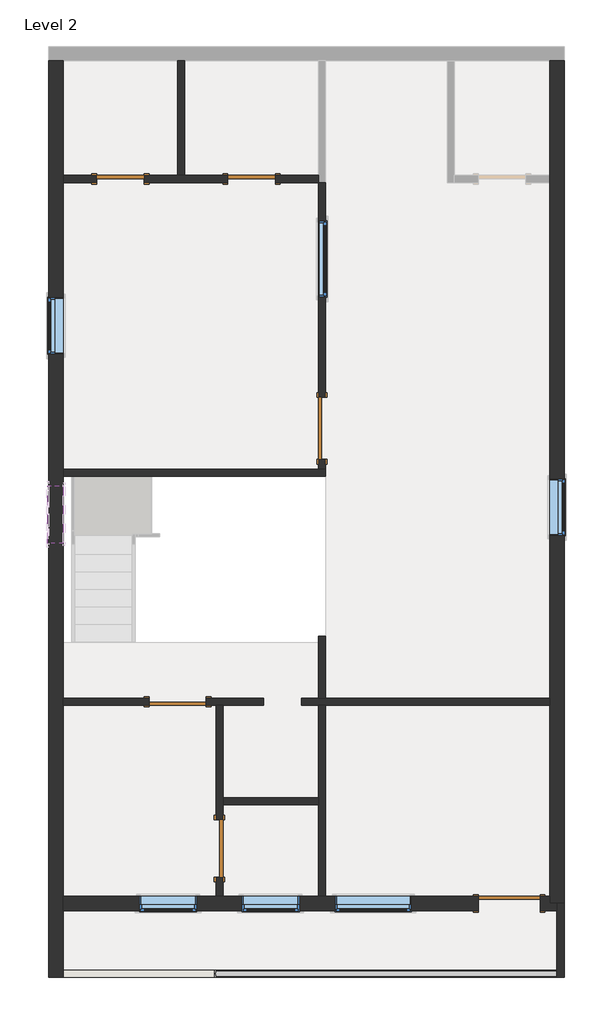
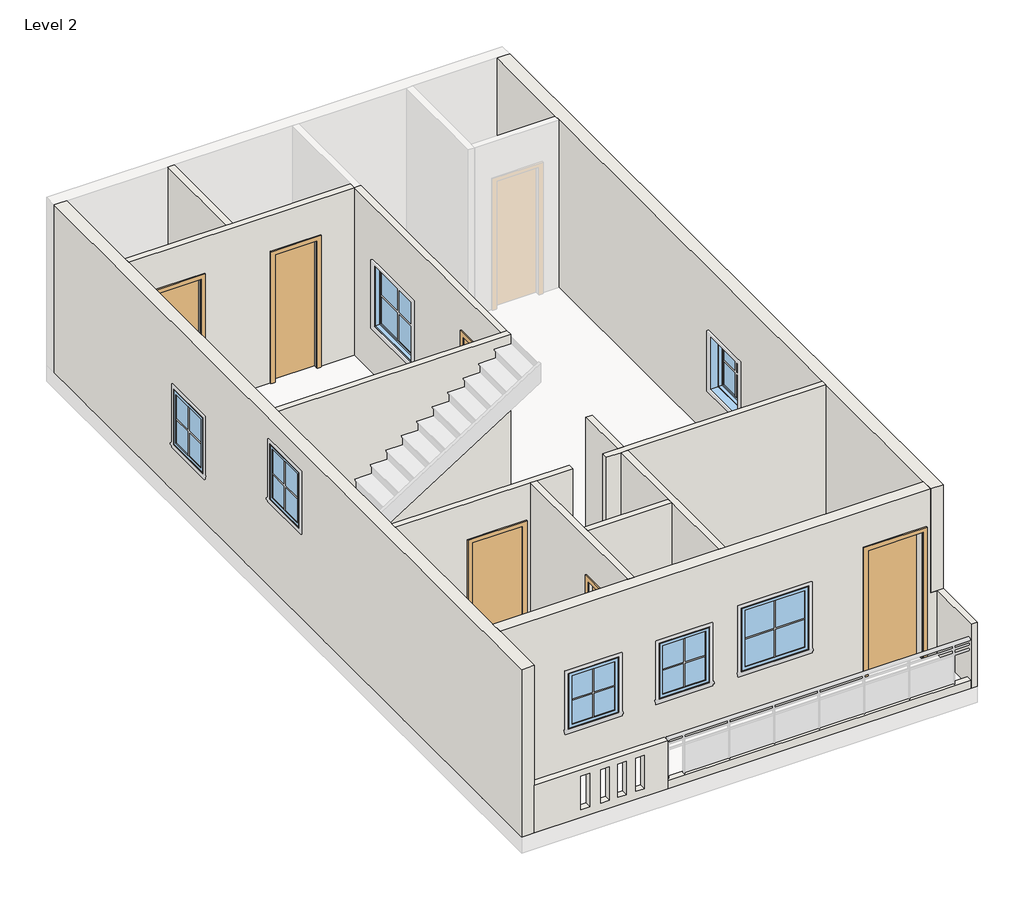
# One storey, part 1 of 2: 15 walls, 7 windows, 6 doors.
"""IFC4 building model written with IfcOpenShell, lengths in millimetres."""

from ifc_helpers import new_model, si_unit, frame, origin, place, context, project, spatial, polyline, outline, extrude, faceted_brep, transform, mapped, element, save
from components import door_02e7543a, door_3ddad2be, single_flush_d2_3_x_7_58d0fc15, door_c9b15bbd, door_019bc352, window_casement_single_left_w_4_x_4_e869003f, window_casement_single_left_w_4_x_4_9640c864, window_cb922c77, window_a1546d9a

model = new_model("IFC4")

# Units and contexts
model_context = context("Model", 3, world=origin())
ifc_project = project(units=[si_unit("LENGTHUNIT", "METRE", prefix="MILLI")], contexts=[model_context])

# Site, building, storey
site = spatial("IfcSite", under=ifc_project)
building = spatial("IfcBuilding", under=site)
storey = spatial("IfcBuildingStorey", under=building, Name="Level 2", Elevation=3200.4)

# Doors
placement = place(None, origin())
door_shape = door_02e7543a(model_context)
element("IfcDoor", 1, ObjectType="Single-Flush : D1 3'3\" X 7'", at=placement, inside=storey, context=model_context, shape_type="MappedRepresentation", body=[
    mapped(door_shape, transform((-6568.6167709, -3138.8637867, 3200.4), x_axis=(1.0, 0.0, 0.0), y_axis=(0.0, 1.0, 0.0), z_axis=(0.0, 0.0, 1.0))),
])
door_2_shape = door_3ddad2be(model_context)
element("IfcDoor", 2, ObjectType="Single-Flush : D1 3'3\" X 7'", at=placement, inside=storey, context=model_context, shape_type="MappedRepresentation", body=[
    mapped(door_2_shape, transform((-9559.4667709, 4443.0362133, 3200.4), x_axis=(0.0, -1.0, 0.0), y_axis=(1.0, 0.0, 0.0), z_axis=(0.0, 0.0, 1.0))),
])
single_flush_d2_3_x_7_shape = single_flush_d2_3_x_7_58d0fc15(model_context)
element("IfcDoor", 3, ObjectType="Single-Flush : D2 3' X 7'", at=placement, inside=storey, context=model_context, shape_type="MappedRepresentation", body=[
    mapped(single_flush_d2_3_x_7_shape, transform((-11864.5167709, 80.5862133, 3200.4), x_axis=(1.0, 0.0, 0.0), y_axis=(0.0, 1.0, 0.0), z_axis=(0.0, 0.0, 1.0))),
])
element("IfcDoor", 4, ObjectType="Single-Flush : D2 3' X 7'", at=placement, inside=storey, context=model_context, shape_type="MappedRepresentation", body=[
    mapped(single_flush_d2_3_x_7_shape, transform((-11197.7667709, -2262.5637867, 3200.4), x_axis=(0.0, 1.0, 0.0), y_axis=(-1.0, 0.0, 0.0), z_axis=(0.0, 0.0, 1.0))),
])
door_3_shape = door_c9b15bbd(model_context)
element("IfcDoor", 5, ObjectType="Single-Flush : D3 2'6\" X 7'", at=placement, inside=storey, context=model_context, shape_type="MappedRepresentation", body=[
    mapped(door_3_shape, transform((-12778.9167709, 8424.4862133, 3200.4), x_axis=(1.0, 0.0, 0.0), y_axis=(0.0, 1.0, 0.0), z_axis=(0.0, 0.0, 1.0))),
])
door_4_shape = door_019bc352(model_context)
element("IfcDoor", 6, ObjectType="Single-Flush : D3 2'6\" X 7'", at=placement, inside=storey, context=model_context, shape_type="MappedRepresentation", body=[
    mapped(door_4_shape, transform((-10683.4167709, 8424.4862133, 3200.4), x_axis=(-1.0, 0.0, 0.0), y_axis=(0.0, -1.0, 0.0), z_axis=(0.0, 0.0, 1.0))),
])

# Walls
element("IfcWall", 7, ObjectType="4.5\" inner wall", at=placement, inside=storey, context=model_context, shape_type="SweptSolid", body=[
    extrude(outline(polyline([(-11864.5167709, 8481.6362133), (-11864.5167709, 10310.4362133), (-11750.2167709, 10310.4362133), (-11750.2167709, 8481.6362133), (-11864.5167709, 8481.6362133)])), frame((0.0, 0.0, 3200.4), z_axis=(0.0, 0.0, 1.0), x_axis=(1.0, 0.0, 0.0)), (0.0, 0.0, 1.0), 3200.4),
])
element("IfcWall", 8, ObjectType="4.5\" inner wall", at=placement, inside=storey, context=model_context, shape_type="Brep", body=[
    faceted_brep([(-11064.4167709, 8481.6362133, 5638.8), (-11064.4167709, 8481.6362133, 3200.4), (-11750.2167709, 8481.6362133, 3200.4), (-11864.5167709, 8481.6362133, 3200.4), (-12397.9167709, 8481.6362133, 3200.4), (-12397.9167709, 8481.6362133, 5638.8), (-13159.9167709, 8481.6362133, 5638.8), (-13159.9167709, 8481.6362133, 3200.4), (-13693.3167709, 8481.6362133, 3200.4), (-13693.3167709, 8481.6362133, 6400.8), (-11864.5167709, 8481.6362133, 6400.8), (-11750.2167709, 8481.6362133, 6400.8), (-9616.6167709, 8481.6362133, 6400.8), (-9616.6167709, 8481.6362133, 3200.4), (-10302.4167709, 8481.6362133, 3200.4), (-10302.4167709, 8481.6362133, 5638.8), (-12397.9167709, 8367.3362133, 3200.4), (-11064.4167709, 8367.3362133, 3200.4), (-11064.4167709, 8367.3362133, 5638.8), (-10302.4167709, 8367.3362133, 5638.8), (-10302.4167709, 8367.3362133, 3200.4), (-9616.6167709, 8367.3362133, 3200.4), (-9616.6167709, 8367.3362133, 6400.8), (-13693.3167709, 8367.3362133, 6400.8), (-13693.3167709, 8367.3362133, 3200.4), (-13159.9167709, 8367.3362133, 3200.4), (-13159.9167709, 8367.3362133, 5638.8), (-12397.9167709, 8367.3362133, 5638.8)], [[[0, 1, 2, 3, 4, 5, 6, 7, 8, 9, 10, 11, 12, 13, 14, 15]], [[16, 17, 18, 19, 20, 21, 22, 23, 24, 25, 26, 27]], [[25, 24, 8, 7]], [[14, 13, 21, 20]], [[4, 3, 2, 1, 17, 16]], [[12, 11, 10, 9, 23, 22]], [[9, 8, 24, 23]], [[13, 12, 22, 21]], [[5, 4, 16, 27]], [[6, 5, 27, 26]], [[7, 6, 26, 25]], [[18, 17, 1, 0]], [[19, 18, 0, 15]], [[20, 19, 15, 14]]]),
])
element("IfcWall", 9, ObjectType="4.5\" inner wall", at=placement, inside=storey, context=model_context, shape_type="Brep", body=[
    faceted_brep([(-13693.3167709, 3681.0362133, 3200.4), (-9502.3167709, 3681.0362133, 3200.4), (-9502.3167709, 3681.0362133, 6400.8), (-13693.3167709, 3681.0362133, 6400.8), (-13693.3167709, 3795.3362133, 3200.4), (-13693.3167709, 3795.3362133, 6400.8), (-9616.6167709, 3795.3362133, 6400.8), (-9502.3167709, 3795.3362133, 6400.8), (-9502.3167709, 3795.3362133, 3200.4), (-9616.6167709, 3795.3362133, 3200.4)], [[[0, 1, 2, 3]], [[4, 5, 6, 7, 8, 9]], [[1, 0, 4, 9, 8]], [[3, 2, 7, 6, 5]], [[0, 3, 5, 4]], [[2, 1, 8, 7]]]),
])
element("IfcWall", 10, ObjectType="4.5\" inner wall", at=placement, inside=storey, context=model_context, shape_type="SweptSolid", body=[
    extrude(outline(polyline([(3947.7362133, 5638.8), (3947.7362133, 3200.4), (3795.3362133, 3200.4), (3795.3362133, 6400.8), (8367.3362133, 6400.8), (8367.3362133, 3200.4), (4938.3362133, 3200.4), (4938.3362133, 5638.8), (3947.7362133, 5638.8)]), holes=[polyline([(6538.5362133, 5334.0), (6538.5362133, 4114.8), (7757.7362133, 4114.8), (7757.7362133, 5334.0), (6538.5362133, 5334.0)])]), frame((-9616.6167709, 0.0, 0.0), z_axis=(1.0, 0.0, 0.0), x_axis=(0.0, 1.0, 0.0)), (0.0, 0.0, 1.0), 114.3),
])
element("IfcWall", 11, ObjectType="4.5\" inner wall", at=placement, inside=storey, context=model_context, shape_type="Brep", body=[
    faceted_brep([(-11407.3167709, 23.4362133, 5638.8), (-11407.3167709, 23.4362133, 3200.4), (-11254.9167709, 23.4362133, 3200.4), (-11140.6167709, 23.4362133, 3200.4), (-10492.9167709, 23.4362133, 3200.4), (-10492.9167709, 23.4362133, 6400.8), (-11140.6167709, 23.4362133, 6400.8), (-11254.9167709, 23.4362133, 6400.8), (-13693.3167709, 23.4362133, 6400.8), (-13693.3167709, 23.4362133, 3200.4), (-12321.7167709, 23.4362133, 3200.4), (-12321.7167709, 23.4362133, 5638.8), (-10492.9167709, 137.7362133, 3200.4), (-11407.3167709, 137.7362133, 3200.4), (-11407.3167709, 137.7362133, 5638.8), (-12321.7167709, 137.7362133, 5638.8), (-12321.7167709, 137.7362133, 3200.4), (-13693.3167709, 137.7362133, 3200.4), (-13693.3167709, 137.7362133, 6400.8), (-10492.9167709, 137.7362133, 6400.8)], [[[0, 1, 2, 3, 4, 5, 6, 7, 8, 9, 10, 11]], [[12, 13, 14, 15, 16, 17, 18, 19]], [[10, 9, 17, 16]], [[4, 3, 2, 1, 13, 12]], [[5, 4, 12, 19]], [[8, 7, 6, 5, 19, 18]], [[9, 8, 18, 17]], [[14, 13, 1, 0]], [[15, 14, 0, 11]], [[16, 15, 11, 10]]]),
])
element("IfcWall", 12, ObjectType="4.5\" inner wall", at=placement, inside=storey, context=model_context, shape_type="Brep", body=[
    faceted_brep([(-11254.9167709, 23.4362133, 3200.4), (-11254.9167709, -1805.3637867, 3200.4), (-11254.9167709, -1805.3637867, 5638.8), (-11254.9167709, -2719.7637867, 5638.8), (-11254.9167709, -2719.7637867, 3200.4), (-11254.9167709, -3024.5637867, 3200.4), (-11254.9167709, -3024.5637867, 6400.8), (-11254.9167709, 23.4362133, 6400.8), (-11140.6167709, -1805.3637867, 5638.8), (-11140.6167709, -1805.3637867, 3200.4), (-11140.6167709, -1564.0637867, 3200.4), (-11140.6167709, -1449.7637867, 3200.4), (-11140.6167709, 23.4362133, 3200.4), (-11140.6167709, 23.4362133, 6400.8), (-11140.6167709, -1449.7637867, 6400.8), (-11140.6167709, -1564.0637867, 6400.8), (-11140.6167709, -3024.5637867, 6400.8), (-11140.6167709, -3024.5637867, 3200.4), (-11140.6167709, -2719.7637867, 3200.4), (-11140.6167709, -2719.7637867, 5638.8)], [[[0, 1, 2, 3, 4, 5, 6, 7]], [[8, 9, 10, 11, 12, 13, 14, 15, 16, 17, 18, 19]], [[18, 17, 5, 4]], [[12, 11, 10, 9, 1, 0]], [[7, 6, 16, 15, 14, 13]], [[6, 5, 17, 16]], [[0, 7, 13, 12]], [[2, 1, 9, 8]], [[3, 2, 8, 19]], [[4, 3, 19, 18]]]),
])
element("IfcWall", 13, ObjectType="4.5\" inner wall", at=placement, inside=storey, context=model_context, shape_type="Brep", body=[
    faceted_brep([(-9502.3167709, 1128.3362133, 3200.4), (-9502.3167709, 1128.3362133, 6400.8), (-9502.3167709, 137.7362133, 6400.8), (-9502.3167709, 137.7362133, 3200.4), (-9616.6167709, 1128.3362133, 6400.8), (-9616.6167709, 1128.3362133, 3200.4), (-9616.6167709, 137.7362133, 3200.4), (-9616.6167709, 137.7362133, 6400.8)], [[[0, 1, 2, 3]], [[4, 5, 6, 7]], [[5, 0, 3, 6]], [[1, 0, 5, 4]], [[1, 4, 7, 2]], [[3, 2, 7, 6]]]),
    faceted_brep([(-9502.3167709, -3024.5637867, 6400.8), (-9502.3167709, -3024.5637867, 3200.4), (-9502.3167709, 23.4362133, 3200.4), (-9502.3167709, 23.4362133, 6400.8), (-9616.6167709, -3024.5637867, 3200.4), (-9616.6167709, -3024.5637867, 6400.8), (-9616.6167709, -1564.0637867, 6400.8), (-9616.6167709, -1449.7637867, 6400.8), (-9616.6167709, 23.4362133, 6400.8), (-9616.6167709, 23.4362133, 3200.4), (-9616.6167709, -1449.7637867, 3200.4), (-9616.6167709, -1564.0637867, 3200.4)], [[[0, 1, 2, 3]], [[4, 5, 6, 7, 8, 9, 10, 11]], [[1, 4, 11, 10, 9, 2]], [[5, 0, 3, 8, 7, 6]], [[1, 0, 5, 4]], [[3, 2, 9, 8]]]),
])
element("IfcWall", 14, ObjectType="4.5\" inner wall", at=placement, inside=storey, context=model_context, shape_type="SweptSolid", body=[
    extrude(outline(polyline([(-9616.6167709, -1564.0637867), (-11140.6167709, -1564.0637867), (-11140.6167709, -1449.7637867), (-9616.6167709, -1449.7637867), (-9616.6167709, -1564.0637867)])), frame((0.0, 0.0, 3200.4), z_axis=(0.0, 0.0, 1.0), x_axis=(1.0, 0.0, 0.0)), (0.0, 0.0, 1.0), 3200.4),
])
element("IfcWall", 15, ObjectType="4.5\" inner wall", at=placement, inside=storey, context=model_context, shape_type="Brep", body=[
    faceted_brep([(-9883.3167709, 23.4362133, 3200.4), (-9616.6167709, 23.4362133, 3200.4), (-9502.3167709, 23.4362133, 3200.4), (-5920.9167709, 23.4362133, 3200.4), (-5920.9167709, 23.4362133, 6400.8), (-9502.3167709, 23.4362133, 6400.8), (-9616.6167709, 23.4362133, 6400.8), (-9883.3167709, 23.4362133, 6400.8), (-9883.3167709, 137.7362133, 3200.4), (-9883.3167709, 137.7362133, 6400.8), (-9616.6167709, 137.7362133, 6400.8), (-9502.3167709, 137.7362133, 6400.8), (-5920.9167709, 137.7362133, 6400.8), (-5920.9167709, 137.7362133, 3200.4), (-9502.3167709, 137.7362133, 3200.4), (-9616.6167709, 137.7362133, 3200.4)], [[[0, 1, 2, 3, 4, 5, 6, 7]], [[8, 9, 10, 11, 12, 13, 14, 15]], [[3, 2, 1, 0, 8, 15, 14, 13]], [[7, 6, 5, 4, 12, 11, 10, 9]], [[0, 7, 9, 8]], [[4, 3, 13, 12]]]),
])
element("IfcWall", 16, ObjectType="4.5\" inner wall", at=placement, inside=storey, context=model_context, shape_type="Brep", body=[
    faceted_brep([(-5806.6167709, -3138.8637867, 3200.4), (-5806.6167709, -3253.1637867, 3200.4), (-5806.6167709, -4205.6637867, 3200.4), (-5806.6167709, -4319.9637867, 3200.4), (-5806.6167709, -4319.9637867, 3352.8), (-5806.6167709, -4319.9637867, 4419.6), (-5806.6167709, -3253.1637867, 4419.6), (-5806.6167709, -3138.8637867, 4419.6), (-5692.3167709, -3138.8637867, 3200.4), (-5692.3167709, -3138.8637867, 4419.6), (-5692.3167709, -3253.1637867, 4419.6), (-5692.3167709, -4319.9637867, 4419.6), (-5692.3167709, -4319.9637867, 3200.4)], [[[0, 1, 2, 3, 4, 5, 6, 7]], [[8, 9, 10, 11, 12]], [[3, 2, 1, 0, 8, 12]], [[7, 6, 5, 11, 10, 9]], [[0, 7, 9, 8]], [[5, 4, 3, 12, 11]]]),
])
element("IfcWall", 17, ObjectType="4.5\" inner wall", at=placement, inside=storey, context=model_context, shape_type="SweptSolid", body=[
    extrude(outline(polyline([(-11280.3167709, -4205.6637867), (-5806.6167709, -4205.6637867), (-5806.6167709, -4319.9637867), (-11280.3167709, -4319.9637867), (-11280.3167709, -4205.6637867)])), frame((0.0, 0.0, 3200.4), z_axis=(0.0, 0.0, 1.0), x_axis=(1.0, 0.0, 0.0)), (0.0, 0.0, 1.0), 152.4),
])
element("IfcWall", 18, ObjectType="4.5\" inner wall", at=placement, inside=storey, context=model_context, shape_type="Brep", body=[
    faceted_brep([(-11280.3167709, -4205.6637867, 3200.4), (-13693.3167709, -4205.6637867, 3200.4), (-13693.3167709, -4205.6637867, 4114.8), (-11280.3167709, -4205.6637867, 4114.8), (-11280.3167709, -4205.6637867, 3352.8), (-12692.2660532, -4205.6637867, 3989.5004539), (-12851.4762568, -4205.6637867, 3989.5004539), (-12851.4762568, -4205.6637867, 3352.8), (-12692.2660532, -4205.6637867, 3352.8), (-12336.6660532, -4205.6637867, 3989.5004539), (-12495.8762568, -4205.6637867, 3989.5004539), (-12495.8762568, -4205.6637867, 3352.8), (-12336.6660532, -4205.6637867, 3352.8), (-12031.8660532, -4205.6637867, 3989.5004539), (-12191.0762568, -4205.6637867, 3989.5004539), (-12191.0762568, -4205.6637867, 3352.8), (-12031.8660532, -4205.6637867, 3352.8), (-11705.3065673, -4205.6637867, 3989.5004539), (-11864.5167709, -4205.6637867, 3989.5004539), (-11864.5167709, -4205.6637867, 3352.8), (-11705.3065673, -4205.6637867, 3352.8), (-11280.3167709, -4319.9637867, 3200.4), (-11280.3167709, -4319.9637867, 3352.8), (-11280.3167709, -4319.9637867, 4114.8), (-13693.3167709, -4319.9637867, 4114.8), (-13693.3167709, -4319.9637867, 3200.4), (-12692.2660532, -4319.9637867, 3989.5004539), (-12692.2660532, -4319.9637867, 3352.8), (-12851.4762568, -4319.9637867, 3352.8), (-12851.4762568, -4319.9637867, 3989.5004539), (-12336.6660532, -4319.9637867, 3989.5004539), (-12336.6660532, -4319.9637867, 3352.8), (-12495.8762568, -4319.9637867, 3352.8), (-12495.8762568, -4319.9637867, 3989.5004539), (-12031.8660532, -4319.9637867, 3989.5004539), (-12031.8660532, -4319.9637867, 3352.8), (-12191.0762568, -4319.9637867, 3352.8), (-12191.0762568, -4319.9637867, 3989.5004539), (-11705.3065673, -4319.9637867, 3989.5004539), (-11705.3065673, -4319.9637867, 3352.8), (-11864.5167709, -4319.9637867, 3352.8), (-11864.5167709, -4319.9637867, 3989.5004539)], [[[0, 1, 2, 3, 4], [5, 6, 7, 8], [9, 10, 11, 12], [13, 14, 15, 16], [17, 18, 19, 20]], [[21, 22, 23, 24, 25], [26, 27, 28, 29], [30, 31, 32, 33], [34, 35, 36, 37], [38, 39, 40, 41]], [[2, 1, 25, 24]], [[1, 0, 21, 25]], [[3, 2, 24, 23]], [[0, 4, 3, 23, 22, 21]], [[6, 5, 26, 29]], [[7, 6, 29, 28]], [[8, 7, 28, 27]], [[5, 8, 27, 26]], [[10, 9, 30, 33]], [[11, 10, 33, 32]], [[12, 11, 32, 31]], [[9, 12, 31, 30]], [[14, 13, 34, 37]], [[15, 14, 37, 36]], [[16, 15, 36, 35]], [[13, 16, 35, 34]], [[18, 17, 38, 41]], [[19, 18, 41, 40]], [[20, 19, 40, 39]], [[17, 20, 39, 38]]]),
])
element("IfcWall", 19, ObjectType="9\" outer wall", at=placement, inside=storey, context=model_context, shape_type="Brep", body=[
    faceted_brep([(-5920.9167709, 10310.4362133, 3200.4), (-5920.9167709, 8481.6362133, 3200.4), (-5920.9167709, 8367.3362133, 3200.4), (-5920.9167709, 137.7362133, 3200.4), (-5920.9167709, 23.4362133, 3200.4), (-5920.9167709, -3024.5637867, 3200.4), (-5920.9167709, -3138.8637867, 3200.4), (-5920.9167709, -3138.8637867, 4419.6), (-5920.9167709, -3253.1637867, 4419.6), (-5920.9167709, -3253.1637867, 6400.8), (-5920.9167709, -3024.5637867, 6400.8), (-5920.9167709, 23.4362133, 6400.8), (-5920.9167709, 137.7362133, 6400.8), (-5920.9167709, 8367.3362133, 6400.8), (-5920.9167709, 8481.6362133, 6400.8), (-5920.9167709, 10310.4362133, 6400.8), (-5920.9167709, 2728.5362133, 5181.6), (-5920.9167709, 2728.5362133, 4114.8), (-5920.9167709, 3642.9362133, 4114.8), (-5920.9167709, 3642.9362133, 5181.6), (-5692.3167709, 10310.4362133, 3200.4), (-5692.3167709, 10310.4362133, 6400.8), (-5692.3167709, -3253.1637867, 6400.8), (-5692.3167709, -3253.1637867, 4419.6), (-5692.3167709, -3138.8637867, 4419.6), (-5692.3167709, -3138.8637867, 3200.4), (-5692.3167709, 2728.5362133, 5181.6), (-5692.3167709, 3642.9362133, 5181.6), (-5692.3167709, 3642.9362133, 4114.8), (-5692.3167709, 2728.5362133, 4114.8), (-5806.6167709, -3138.8637867, 3200.4), (-5806.6167709, -3138.8637867, 4419.6), (-5806.6167709, -3253.1637867, 4419.6)], [[[0, 1, 2, 3, 4, 5, 6, 7, 8, 9, 10, 11, 12, 13, 14, 15], [16, 17, 18, 19]], [[20, 21, 22, 23, 24, 25], [26, 27, 28, 29]], [[6, 5, 4, 3, 2, 1, 0, 20, 25, 30]], [[15, 14, 13, 12, 11, 10, 9, 22, 21]], [[0, 15, 21, 20]], [[7, 6, 30, 25, 24, 31]], [[23, 32, 8, 7, 31, 24]], [[9, 8, 32, 23, 22]], [[17, 16, 26, 29]], [[18, 17, 29, 28]], [[19, 18, 28, 27]], [[16, 19, 27, 26]]]),
])
element("IfcWall", 20, ObjectType="9\" outer wall", at=placement, inside=storey, context=model_context, shape_type="Brep", body=[
    faceted_brep([(-13693.3167709, -4319.9637867, 3200.4), (-13693.3167709, -4205.6637867, 3200.4), (-13693.3167709, -3253.1637867, 3200.4), (-13693.3167709, -3024.5637867, 3200.4), (-13693.3167709, 23.4362133, 3200.4), (-13693.3167709, 137.7362133, 3200.4), (-13693.3167709, 3681.0362133, 3200.4), (-13693.3167709, 3795.3362133, 3200.4), (-13693.3167709, 8367.3362133, 3200.4), (-13693.3167709, 8481.6362133, 3200.4), (-13693.3167709, 10310.4362133, 3200.4), (-13693.3167709, 10310.4362133, 6400.8), (-13693.3167709, 8481.6362133, 6400.8), (-13693.3167709, 8367.3362133, 6400.8), (-13693.3167709, 3795.3362133, 6400.8), (-13693.3167709, 3681.0362133, 6400.8), (-13693.3167709, 137.7362133, 6400.8), (-13693.3167709, 23.4362133, 6400.8), (-13693.3167709, -3024.5637867, 6400.8), (-13693.3167709, -3253.1637867, 6400.8), (-13693.3167709, -4319.9637867, 6400.8), (-13693.3167709, -4319.9637867, 4114.8), (-13693.3167709, 6538.5362133, 5181.6), (-13693.3167709, 6538.5362133, 4114.8), (-13693.3167709, 5624.1362133, 4114.8), (-13693.3167709, 5624.1362133, 5181.6), (-13693.3167709, 3528.6362133, 5961.0278271), (-13693.3167709, 3528.6362133, 4894.2278271), (-13693.3167709, 2614.2362133, 4894.2278271), (-13693.3167709, 2614.2362133, 5961.0278271), (-13921.9167709, -4319.9637867, 3200.4), (-13921.9167709, -4319.9637867, 6400.8), (-13921.9167709, 10310.4362133, 6400.8), (-13921.9167709, 10310.4362133, 3200.4), (-13921.9167709, 6538.5362133, 5181.6), (-13921.9167709, 5624.1362133, 5181.6), (-13921.9167709, 5624.1362133, 4114.8), (-13921.9167709, 6538.5362133, 4114.8), (-13921.9167709, 3528.6362133, 5961.0278271), (-13921.9167709, 2614.2362133, 5961.0278271), (-13921.9167709, 2614.2362133, 4894.2278271), (-13921.9167709, 3528.6362133, 4894.2278271)], [[[0, 1, 2, 3, 4, 5, 6, 7, 8, 9, 10, 11, 12, 13, 14, 15, 16, 17, 18, 19, 20, 21], [22, 23, 24, 25], [26, 27, 28, 29]], [[30, 31, 32, 33], [34, 35, 36, 37], [38, 39, 40, 41]], [[10, 9, 8, 7, 6, 5, 4, 3, 2, 1, 0, 30, 33]], [[20, 19, 18, 17, 16, 15, 14, 13, 12, 11, 32, 31]], [[11, 10, 33, 32]], [[0, 21, 20, 31, 30]], [[23, 22, 34, 37]], [[24, 23, 37, 36]], [[25, 24, 36, 35]], [[22, 25, 35, 34]], [[27, 26, 38, 41]], [[28, 27, 41, 40]], [[29, 28, 40, 39]], [[26, 29, 39, 38]]]),
])
element("IfcWall", 21, ObjectType="9\" outer wall", at=placement, inside=storey, context=model_context, shape_type="Brep", body=[
    faceted_brep([(-5920.9167709, -3024.5637867, 3200.4), (-6073.3167709, -3024.5637867, 3200.4), (-6073.3167709, -3024.5637867, 5638.8), (-7063.9167709, -3024.5637867, 5638.8), (-7063.9167709, -3024.5637867, 3200.4), (-9502.3167709, -3024.5637867, 3200.4), (-9616.6167709, -3024.5637867, 3200.4), (-11140.6167709, -3024.5637867, 3200.4), (-11254.9167709, -3024.5637867, 3200.4), (-13693.3167709, -3024.5637867, 3200.4), (-13693.3167709, -3024.5637867, 6400.8), (-11254.9167709, -3024.5637867, 6400.8), (-11140.6167709, -3024.5637867, 6400.8), (-9616.6167709, -3024.5637867, 6400.8), (-9502.3167709, -3024.5637867, 6400.8), (-5920.9167709, -3024.5637867, 6400.8), (-5920.9167709, -3024.5637867, 4419.6), (-8130.7167709, -3024.5637867, 5334.0), (-9349.9167709, -3024.5637867, 5334.0), (-9349.9167709, -3024.5637867, 4114.8), (-8130.7167709, -3024.5637867, 4114.8), (-9921.4167709, -3024.5637867, 5181.6), (-10835.8167709, -3024.5637867, 5181.6), (-10835.8167709, -3024.5637867, 4114.8), (-9921.4167709, -3024.5637867, 4114.8), (-11559.7167709, -3024.5637867, 5181.6), (-12474.1167709, -3024.5637867, 5181.6), (-12474.1167709, -3024.5637867, 4114.8), (-11559.7167709, -3024.5637867, 4114.8), (-6073.3167709, -3253.1637867, 5638.8), (-6073.3167709, -3253.1637867, 3200.4), (-5806.6167709, -3253.1637867, 3200.4), (-5806.6167709, -3253.1637867, 4419.6), (-5920.9167709, -3253.1637867, 4419.6), (-5920.9167709, -3253.1637867, 6400.8), (-13693.3167709, -3253.1637867, 6400.8), (-13693.3167709, -3253.1637867, 3200.4), (-7063.9167709, -3253.1637867, 3200.4), (-7063.9167709, -3253.1637867, 5638.8), (-8130.7167709, -3253.1637867, 5334.0), (-8130.7167709, -3253.1637867, 4114.8), (-9349.9167709, -3253.1637867, 4114.8), (-9349.9167709, -3253.1637867, 5334.0), (-9921.4167709, -3253.1637867, 5181.6), (-9921.4167709, -3253.1637867, 4114.8), (-10835.8167709, -3253.1637867, 4114.8), (-10835.8167709, -3253.1637867, 5181.6), (-11559.7167709, -3253.1637867, 5181.6), (-11559.7167709, -3253.1637867, 4114.8), (-12474.1167709, -3253.1637867, 4114.8), (-12474.1167709, -3253.1637867, 5181.6), (-5920.9167709, -3138.8637867, 3200.4), (-5806.6167709, -3138.8637867, 3200.4), (-5920.9167709, -3138.8637867, 4419.6), (-5806.6167709, -3138.8637867, 4419.6)], [[[0, 1, 2, 3, 4, 5, 6, 7, 8, 9, 10, 11, 12, 13, 14, 15, 16], [17, 18, 19, 20], [21, 22, 23, 24], [25, 26, 27, 28]], [[29, 30, 31, 32, 33, 34, 35, 36, 37, 38], [39, 40, 41, 42], [43, 44, 45, 46], [47, 48, 49, 50]], [[37, 36, 9, 8, 7, 6, 5, 4]], [[31, 30, 1, 0, 51, 52]], [[15, 14, 13, 12, 11, 10, 35, 34]], [[10, 9, 36, 35]], [[40, 39, 17, 20]], [[41, 40, 20, 19]], [[42, 41, 19, 18]], [[39, 42, 18, 17]], [[44, 43, 21, 24]], [[45, 44, 24, 23]], [[46, 45, 23, 22]], [[43, 46, 22, 21]], [[48, 47, 25, 28]], [[49, 48, 28, 27]], [[50, 49, 27, 26]], [[47, 50, 26, 25]], [[2, 1, 30, 29]], [[3, 2, 29, 38]], [[4, 3, 38, 37]], [[53, 33, 32, 54]], [[0, 16, 53, 51]], [[16, 15, 34, 33, 53]], [[53, 54, 52, 51]], [[54, 32, 31, 52]]]),
])

# Windows
window_casement_single_left_w_4_x_4_shape = window_casement_single_left_w_4_x_4_e869003f(model_context)
element("IfcWindow", 22, ObjectType="Window-Casement-Single_Left : W 4' X 4'", at=placement, inside=storey, context=model_context, shape_type="MappedRepresentation", body=[
    mapped(window_casement_single_left_w_4_x_4_shape, transform((-8740.3167709, -3138.8637867, 3200.4), x_axis=(1.0, 0.0, 0.0), y_axis=(0.0, 1.0, 0.0), z_axis=(0.0, 0.0, 1.0))),
])
window_casement_single_left_w_4_x_4_2_shape = window_casement_single_left_w_4_x_4_9640c864(model_context)
element("IfcWindow", 23, ObjectType="Window-Casement-Single_Left : W 4' X 4'", at=placement, inside=storey, context=model_context, shape_type="MappedRepresentation", body=[
    mapped(window_casement_single_left_w_4_x_4_2_shape, transform((-9559.4667709, 7148.1362133, 3200.4), x_axis=(0.0, -1.0, 0.0), y_axis=(1.0, 0.0, 0.0), z_axis=(0.0, 0.0, 1.0))),
])
window_shape = window_cb922c77(model_context)
element("IfcWindow", 24, ObjectType="Window-Casement-Single_Left : W3 3' X 3'6\"", at=placement, inside=storey, context=model_context, shape_type="MappedRepresentation", body=[
    mapped(window_shape, transform((-10378.6167709, -3138.8637867, 3200.4), x_axis=(1.0, 0.0, 0.0), y_axis=(0.0, 1.0, 0.0), z_axis=(0.0, 0.0, 1.0))),
])
element("IfcWindow", 25, ObjectType="Window-Casement-Single_Left : W3 3' X 3'6\"", at=placement, inside=storey, context=model_context, shape_type="MappedRepresentation", body=[
    mapped(window_shape, transform((-12016.9167709, -3138.8637867, 3200.4), x_axis=(1.0, 0.0, 0.0), y_axis=(0.0, 1.0, 0.0), z_axis=(0.0, 0.0, 1.0))),
])
window_2_shape = window_a1546d9a(model_context)
element("IfcWindow", 26, ObjectType="Window-Casement-Single_Left : W3 3' X 3'6\"", at=placement, inside=storey, context=model_context, shape_type="MappedRepresentation", body=[
    mapped(window_2_shape, transform((-13807.6167709, 6081.3362133, 3200.4), x_axis=(0.0, 1.0, 0.0), y_axis=(-1.0, 0.0, 0.0), z_axis=(0.0, 0.0, 1.0))),
])
element("IfcWindow", 27, ObjectType="Window-Casement-Single_Left : W3 3' X 3'6\"", at=placement, inside=storey, context=model_context, shape_type="MappedRepresentation", body=[
    mapped(window_2_shape, transform((-13807.6167709, 3071.4362133, 3979.8278271), x_axis=(0.0, 1.0, 0.0), y_axis=(-1.0, 0.0, 0.0), z_axis=(0.0, 0.0, 1.0))),
])
element("IfcWindow", 28, ObjectType="Window-Casement-Single_Left : W3 3' X 3'6\"", at=placement, inside=storey, context=model_context, shape_type="MappedRepresentation", body=[
    mapped(window_2_shape, transform((-5806.6167709, 3185.7362133, 3200.4), x_axis=(0.0, -1.0, 0.0), y_axis=(1.0, 0.0, 0.0), z_axis=(0.0, 0.0, 1.0))),
])

save(model, "model.ifc")

# Revit data of these elements
# Type "Single-Flush : D1 3'3\" X 7'"
#   Type Mark = "9"
#   Construction Type Id = "MDOOR"
#   Assembly Code = "C1020"
#   Analytic Construction = "Metal"
#   Thickness = 0' - 2"
#   Heat Transfer Coefficient (U) = 0.651978 BTU/(h·ft²·°F)
#   Height = 8' - 0"
#   Trim Projection Ext = 0' - 1"
#   Trim Projection Int = 0' - 1"
#   Trim Width = 0' - 3"
#   Width = 3' - 3"
#   Define Thermal Properties by = 1
#   Door Material = Door - Panel
#   Frame Material = Door - Frame
#   Visual Light Transmittance = 0
#   Solar Heat Gain Coefficient = 0
#   Function = (empty or 0)
#   Wall Closure = (empty or 0)
# Type "Single-Flush : D2 3' X 7'"
#   Type Mark = "10"
#   Construction Type Id = "MDOOR"
#   Assembly Code = "C1020"
#   Analytic Construction = "Metal"
#   Thickness = 0' - 2"
#   Heat Transfer Coefficient (U) = 0.651978 BTU/(h·ft²·°F)
#   Height = 8' - 0"
#   Trim Projection Ext = 0' - 1"
#   Trim Projection Int = 0' - 1"
#   Trim Width = 0' - 3"
#   Width = 3' - 0"
#   Define Thermal Properties by = 1
#   Door Material = Door - Panel
#   Frame Material = Door - Frame
#   Visual Light Transmittance = 0
#   Solar Heat Gain Coefficient = 0
#   Function = (empty or 0)
#   Wall Closure = (empty or 0)
# Type "Single-Flush : D3 2'6\" X 7'"
#   Type Mark = "11"
#   Construction Type Id = "MDOOR"
#   Assembly Code = "C1020"
#   Analytic Construction = "Metal"
#   Thickness = 0' - 2"
#   Heat Transfer Coefficient (U) = 0.651978 BTU/(h·ft²·°F)
#   Height = 8' - 0"
#   Trim Projection Ext = 0' - 1"
#   Trim Projection Int = 0' - 1"
#   Trim Width = 0' - 3"
#   Width = 2' - 6"
#   Define Thermal Properties by = 1
#   Door Material = Door - Panel
#   Frame Material = Door - Frame
#   Visual Light Transmittance = 0
#   Solar Heat Gain Coefficient = 0
#   Function = (empty or 0)
#   Wall Closure = (empty or 0)
# Type "4.5\" inner wall"
#   Assembly Code = "B2010"
#   Layers, outside or top first: 0' - 4 1/2" no material (function 1)
# Type "9\" outer wall"
#   Assembly Code = "B2010"
#   Layers, outside or top first: 0' - 9" no material (function 1)
# Type "Window-Casement-Single_Left : W 4' X 4'"
#   Type Mark = "19"
#   Fire Rating = "0.5h"
#   Assembly Code = "B2020100"
#   Analytic Construction = "Double glazing - domestic"
#   Window Inset [instance default] = 0' - 0"
#   Wall Thickness [instance default] = 0' - 6"
#   Visual Light Transmittance = 0.81
#   Thermal Resistance (R) = 1.8146 (h·ft²·°F)/BTU
#   Solar Heat Gain Coefficient = 0.76
#   Rough Width = 4' - 0 1/2"
#   Rough Height = 4' - 0 1/2"
#   Interior Wall Closure [instance default] = 0' - 2 1/4"
#   Height = 4' - 0"
#   Heat Transfer Coefficient (U) = 0.5511 BTU/(h·ft²·°F)
#   Frame Extension [instance default] = 0' - 0 1/4"
#   Exterior Wall Closure [instance default] = 0' - 1 1/4"
#   Extension Jamb [instance default] = 0' - 2 1/4"
#   Default Sill Height = 3' - 0"
#   Width = 4' - 0"
#   Muntin Visibility = yes
#   Interior Trim Visibility [instance default] = yes
#   Exterior Trim Visibility [instance default] = yes
#   Extension Jamb Visibility [instance default] = yes
#   Muntin Pattern = Muntin Pattern_2x2 : Muntin Pattern_2x2
#   Interior Trim Material = Wood - Stained
#   Interior Trim = Trim-Window-Interior-Flat : Picture Frame
#   Interior Frame Material = Wood - Stained
#   Glass Panel Material = Glass
#   Exterior Trim Material = Clad - White
#   Exterior Trim = Trim-Window-Exterior-Flat : with Sill
#   Exterior Frame Material = Clad - White
#   Wall Closure = (empty or 0)
# Type "Window-Casement-Single_Left : W3 3' X 3'6\""
#   Type Mark = "20"
#   Fire Rating = "0.5h"
#   Assembly Code = "B2020100"
#   Analytic Construction = "Double glazing - domestic"
#   Window Inset [instance default] = 0' - 0"
#   Wall Thickness [instance default] = 0' - 6"
#   Visual Light Transmittance = 0.81
#   Thermal Resistance (R) = 1.8146 (h·ft²·°F)/BTU
#   Solar Heat Gain Coefficient = 0.76
#   Rough Width = 3' - 0 1/2"
#   Rough Height = 3' - 6 1/2"
#   Interior Wall Closure [instance default] = 0' - 2 1/4"
#   Height = 3' - 6"
#   Heat Transfer Coefficient (U) = 0.5511 BTU/(h·ft²·°F)
#   Frame Extension [instance default] = 0' - 0 1/4"
#   Exterior Wall Closure [instance default] = 0' - 1 1/4"
#   Extension Jamb [instance default] = 0' - 2 1/4"
#   Default Sill Height = 3' - 0"
#   Width = 3' - 0"
#   Muntin Visibility = yes
#   Interior Trim Visibility [instance default] = yes
#   Exterior Trim Visibility [instance default] = yes
#   Extension Jamb Visibility [instance default] = yes
#   Muntin Pattern = Muntin Pattern_2x2 : Muntin Pattern_2x2
#   Interior Trim Material = Wood - Stained
#   Interior Trim = Trim-Window-Interior-Flat : Picture Frame
#   Interior Frame Material = Wood - Stained
#   Glass Panel Material = Glass
#   Exterior Trim Material = Clad - White
#   Exterior Trim = Trim-Window-Exterior-Flat : with Sill
#   Exterior Frame Material = Clad - White
#   Wall Closure = (empty or 0)
# Elements 1, 2 (IfcDoor, "Single-Flush : D1 3'3\" X 7'")
#   Phase Created = New Construction
#   Materials on its faces: "Door - Frame", "Door - Panel"
# Elements 3, 4 (IfcDoor, "Single-Flush : D2 3' X 7'")
#   Phase Created = New Construction
#   Materials on its faces: "Door - Frame", "Door - Panel"
# Elements 5, 6 (IfcDoor, "Single-Flush : D3 2'6\" X 7'")
#   Phase Created = New Construction
#   Materials on its faces: "Door - Frame", "Door - Panel"
# Elements 7, 8, 9, 10, 11, 12, 13, 14, 15 (IfcWall, "4.5\" inner wall")
#   Top Offset = 0' - 0"
#   Base Offset = 0' - 0"
#   wall height = 10' - 6"
#   Phase Created = New Construction
#   Base Constraint = Level 2
#   Top Constraint = Level 3
#   Materials on its faces: "Default Wall"
# Element 16 (IfcWall, "4.5\" inner wall")
#   Top Offset = 0' - 0"
#   Base Offset = 0' - 0"
#   Unconnected Height = 4' - 0"
#   wall height = 4' - 0"
#   Phase Created = New Construction
#   Base Constraint = Level 2
#   Materials on its faces: "Default Wall"
# Element 17 (IfcWall, "4.5\" inner wall")
#   Top Offset = 0' - 0"
#   Base Offset = 0' - 0"
#   Unconnected Height = 0' - 6"
#   wall height = 0' - 6"
#   Phase Created = New Construction
#   Base Constraint = Level 2
#   Materials on its faces: "Default Wall"
# Element 18 (IfcWall, "4.5\" inner wall")
#   Top Offset = 0' - 0"
#   Base Offset = 0' - 0"
#   Unconnected Height = 3' - 0"
#   wall height = 3' - 0"
#   Phase Created = New Construction
#   Base Constraint = Level 2
#   Materials on its faces: "Default Wall"
# Elements 19, 20, 21 (IfcWall, "9\" outer wall")
#   Top Offset = 0' - 0"
#   Base Offset = 0' - 0"
#   wall height = 10' - 6"
#   Phase Created = New Construction
#   Base Constraint = Level 2
#   Top Constraint = Level 3
#   Materials on its faces: "Default Wall"
# Element 22 (IfcWindow, "Window-Casement-Single_Left : W 4' X 4'")
#   Mark = "8"
#   Window Inset = 0' - 0"
#   Interior Wall Closure = 0' - 2 1/4"
#   Frame Extension = 0' - 0 1/4"
#   Exterior Wall Closure = 0' - 1 1/4"
#   Interior Trim Visibility = yes
#   Exterior Trim Visibility = yes
#   Phase Created = New Construction
#   Materials on its faces: "Wood - Stained", "Glass", "Clad - White"
# Element 23 (IfcWindow, "Window-Casement-Single_Left : W 4' X 4'")
#   Mark = "11"
#   Window Inset = 0' - 0"
#   Interior Wall Closure = 0' - 2 1/4"
#   Frame Extension = 0' - 0 1/4"
#   Exterior Wall Closure = 0' - 1 1/4"
#   Interior Trim Visibility = yes
#   Exterior Trim Visibility = yes
#   Phase Created = New Construction
#   Materials on its faces: "Wood - Stained", "Glass", "Clad - White"
# Element 24 (IfcWindow, "Window-Casement-Single_Left : W3 3' X 3'6\"")
#   Mark = "9"
#   Window Inset = 0' - 0"
#   Interior Wall Closure = 0' - 2 1/4"
#   Frame Extension = 0' - 0 1/4"
#   Exterior Wall Closure = 0' - 1 1/4"
#   Interior Trim Visibility = yes
#   Exterior Trim Visibility = yes
#   Phase Created = New Construction
#   Materials on its faces: "Wood - Stained", "Glass", "Clad - White"
# Element 25 (IfcWindow, "Window-Casement-Single_Left : W3 3' X 3'6\"")
#   Mark = "10"
#   Window Inset = 0' - 0"
#   Interior Wall Closure = 0' - 2 1/4"
#   Frame Extension = 0' - 0 1/4"
#   Exterior Wall Closure = 0' - 1 1/4"
#   Interior Trim Visibility = yes
#   Exterior Trim Visibility = yes
#   Phase Created = New Construction
#   Materials on its faces: "Wood - Stained", "Glass", "Clad - White"
# Element 26 (IfcWindow, "Window-Casement-Single_Left : W3 3' X 3'6\"")
#   Mark = "15"
#   Window Inset = 0' - 0"
#   Interior Wall Closure = 0' - 2 1/4"
#   Frame Extension = 0' - 0 1/4"
#   Exterior Wall Closure = 0' - 1 1/4"
#   Interior Trim Visibility = yes
#   Exterior Trim Visibility = yes
#   Phase Created = New Construction
#   Materials on its faces: "Wood - Stained", "Glass", "Clad - White"
# Element 27 (IfcWindow, "Window-Casement-Single_Left : W3 3' X 3'6\"")
#   Mark = "16"
#   Window Inset = 0' - 0"
#   Interior Wall Closure = 0' - 2 1/4"
#   Frame Extension = 0' - 0 1/4"
#   Exterior Wall Closure = 0' - 1 1/4"
#   Interior Trim Visibility = yes
#   Exterior Trim Visibility = yes
#   Phase Created = New Construction
#   Materials on its faces: "Wood - Stained", "Glass", "Clad - White"
# Element 28 (IfcWindow, "Window-Casement-Single_Left : W3 3' X 3'6\"")
#   Mark = "17"
#   Window Inset = 0' - 0"
#   Interior Wall Closure = 0' - 2 1/4"
#   Frame Extension = 0' - 0 1/4"
#   Exterior Wall Closure = 0' - 1 1/4"
#   Interior Trim Visibility = yes
#   Exterior Trim Visibility = yes
#   Phase Created = New Construction
#   Materials on its faces: "Wood - Stained", "Glass", "Clad - White"
# Materials
#   "Door - Panel": class "Wood", colour RGB 210 159 95, transparency 0, Cost = 0
#   "Door - Frame": colour RGB 118 70 51, transparency 0, Cost = 0
#   "Wood - Stained": class "Wood", colour RGB 224 178 126, transparency 0, Cost = 0
#   "Glass": class "Glass", colour RGB 0 128 192, transparency 0.75, Description = "Soda Lime Glass", Cost = 0
#   "Clad - White": class "Wood", colour RGB 242 242 238, transparency 0, Cost = 0
#   "Default Wall": colour RGB 128 128 128, transparency 0, Cost = 0
